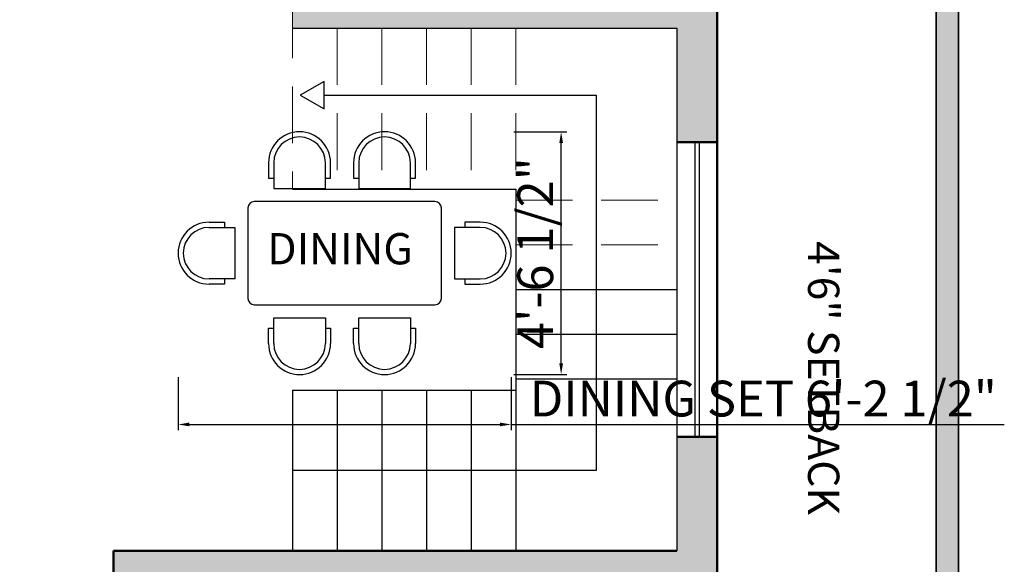
# Model space of a CAD drawing. Units: inches. Extents: x 3008 to 4088, y 1255 to 2137.
# Tile 10 of 30: x 3310 to 3530, y 1665 to 1787. Entities that reach past the tile are written whole.
import ezdxf

# ---------------------------------------------------------------- set-up
doc = ezdxf.new("R2010")
doc.units = ezdxf.units.IN
doc.linetypes.add('DASHED', pattern=[19.05, 12.7, -6.35])
for name, color, linetype, lineweight in [('A-ANNO-DIMS', 2, 'Continuous', 18), ('A-ANNO-TEXT', 7, 'Continuous', 18), ('A-AREA-IDEN', 7, 'Continuous', 18), ('A-FLOR-STRS', 3, 'Continuous', 25), ('A-FLOR-STRS-OVHD', 3, 'DASHED', 18), ('A-FURN', 8, 'Continuous', 18), ('A-GLAZ', 4, 'Continuous', 25), ('A-WALL', 7, 'Continuous', 50), ('A-WALL-PATT', 8, 'Continuous', 13), ('C-PROP', 1, 'Continuous', 35), ('C-PROP-PATT', 9, 'Continuous', 13)]:
    doc.layers.add(name, color=color, linetype=linetype, lineweight=lineweight)
doc.layers.add('NOI THAT', color=42, linetype='Continuous')
doc.styles.get("Standard").update_dxf_attribs({"font": 'arial.ttf'})
doc.dimstyles.new('ISO-25', dxfattribs={"dimtxt": 8, "dimasz": 2.5, "dimexe": 1.25, "dimexo": 0.625, "dimtad": 1, "dimdec": 1, "dimlunit": 3, "dimtxsty": 'Standard', "dimcen": 2.5, "dimadec": 0, "dimazin": 0, "dimtfac": 1, "dimtdec": 1, "dimtmove": 0, "dimatfit": 3, "dimfxl": 1, "dimarcsym": 0})

# ---------------------------------------------------------------- blocks, each defined once
blk = doc.blocks.new('A$C3F0C2877')
at = {"layer": 'NOI THAT'}
for p, q in [((700, 1640), (700, 1520)), ((740, 1640), (740, 1440)), ((1140, 1440), (1140, 1640)), ((1180, 1520), (1180, 1640)), ((1358.3, 1640), (1358.3, 1520)), ((1398.3, 1640), (1398.3, 1440)), ((1798.3, 1440), (1798.3, 1640)), ((1838.3, 1520), (1838.3, 1640)), ((700, 1520), (740, 1520)), ((1140, 1520), (1180, 1520)), ((1358.3, 1520), (1398.3, 1520)), ((1798.3, 1520), (1838.3, 1520)), ((740, 1440), (1140, 1440)), ((1398.3, 1440), (1798.3, 1440)), ((1988.3, 1340), (590, 1340)), ((540, 1290), (540, 590)), ((2038.3, 590), (2038.3, 1290)), ((240, 1180), (360, 1180)), ((360, 1180), (360, 1140)), ((2338.6, 1180), (2218.6, 1180)), ((2218.6, 1180), (2218.6, 1140)), ((240, 1140), (440, 1140)), ((440, 1140), (440, 740)), ((2138.6, 1140), (2138.6, 740)), ((2338.6, 1140), (2138.6, 1140)), ((440, 740), (240, 740)), ((360, 700), (240, 700)), ((360, 740), (360, 700)), ((2138.6, 740), (2338.6, 740)), ((2218.6, 740), (2218.6, 700)), ((2218.6, 700), (2338.6, 700)), ((590, 540), (1988.3, 540)), ((740, 440), (1140, 440)), ((740, 240), (740, 440)), ((1140, 440), (1140, 240)), ((1398.3, 440), (1798.3, 440)), ((1398.3, 240), (1398.3, 440)), ((1798.3, 440), (1798.3, 240)), ((700, 360), (740, 360)), ((700, 240), (700, 360)), ((1140, 360), (1180, 360)), ((1180, 360), (1180, 240)), ((1358.3, 360), (1398.3, 360)), ((1358.3, 240), (1358.3, 360)), ((1798.3, 360), (1838.3, 360)), ((1838.3, 360), (1838.3, 240))]:
    blk.add_line(p, q, dxfattribs=at)
for centre, radius, start, end in [((940, 1640), 240, 0, 180), ((940, 1640), 200, 0, 180), ((1598.3, 1640), 240, 0, 180), ((1598.3, 1640), 200, 0, 180), ((590, 1290), 50, 90, 180), ((1988.3, 1290), 50, 0, 90), ((240, 940), 240, 90, 270), ((2338.6, 940), 240, 270, 90), ((240, 940), 200, 90, 270), ((2338.6, 940), 200, 270, 90), ((590, 590), 50, 180, 270), ((1988.3, 590), 50, 270, 0), ((940, 240), 240, 180, 0), ((940, 240), 200, 180, 0), ((1598.3, 240), 240, 180, 0), ((1598.3, 240), 200, 180, 0)]:
    blk.add_arc(centre, radius, start, end, dxfattribs=at)
blk = doc.blocks.new('*D65')
at = {"layer": 'A-ANNO-DIMS', "color": 0, "lineweight": -2, "transparency": 16777216}
for p, q in [((3345.11, 1706.82), (3345.11, 1695.02)), ((3419.62, 1706.82), (3419.62, 1695.02)), ((3347.61, 1696.27), (3417.12, 1696.27)), ((3419.62, 1696.27), (3529.94, 1696.27))]:
    blk.add_line(p, q, dxfattribs=at)
at = {"layer": 'A-ANNO-DIMS', "color": 0, "transparency": 16777216}
for points in [[(3347.61, 1696.69), (3347.61, 1695.86), (3345.11, 1696.27)], [(3417.12, 1696.69), (3417.12, 1695.86), (3419.62, 1696.27)]]:
    blk.add_solid(points, dxfattribs=at)
at = {"layer": 'Defpoints', "color": 0, "transparency": 16777216}
for p in [(3345.11, 1707.45), (3419.62, 1707.45), (3419.62, 1696.27)]:
    blk.add_point(p, dxfattribs=at)
at = {"layer": 'A-ANNO-DIMS', "color": 0, "transparency": 16777216, "insert": (3476.03, 1701.03), "char_height": 8, "attachment_point": 5}
blk.add_mtext('DINING SET 6\'-2 1/2"', dxfattribs=at)
blk = doc.blocks.new('*D66')
at = {"layer": 'A-ANNO-DIMS', "color": 0, "lineweight": -2, "transparency": 16777216}
for p, q in [((3420.25, 1761.77), (3432.05, 1761.77)), ((3430.8, 1709.95), (3430.8, 1759.27)), ((3420.25, 1707.45), (3432.05, 1707.45))]:
    blk.add_line(p, q, dxfattribs=at)
at = {"layer": 'A-ANNO-DIMS', "color": 0, "transparency": 16777216}
for points in [[(3430.38, 1759.27), (3431.21, 1759.27), (3430.8, 1761.77)], [(3430.38, 1709.95), (3431.21, 1709.95), (3430.8, 1707.45)]]:
    blk.add_solid(points, dxfattribs=at)
at = {"layer": 'Defpoints', "color": 0, "transparency": 16777216}
for p in [(3419.62, 1761.77), (3430.8, 1761.77), (3419.62, 1707.45)]:
    blk.add_point(p, dxfattribs=at)
at = {"layer": 'A-ANNO-DIMS', "color": 0, "transparency": 16777216, "insert": (3426.04, 1734.61), "char_height": 8, "attachment_point": 5, "rotation": 90}
blk.add_mtext('4\'-6 1/2"', dxfattribs=at)

msp = doc.modelspace()

# ---------------------------------------------------------------- hatches: boundary and pattern name
at = {"layer": 'A-WALL-PATT'}
h = msp.add_hatch(color=256, dxfattribs=at)
h.dxf.hatch_style = 1
h.paths.add_polyline_path([(3102.67, 1625.97), (3093.67, 1625.97), (3093.67, 1540.97), (3102.67, 1540.97)])
h.paths.add_polyline_path([(3102.67, 1784.97), (3252.67, 1784.97), (3252.67, 1790.97), (3102.67, 1790.97), (3102.67, 1892.97), (3093.67, 1892.97), (3093.67, 1667.97), (3102.67, 1667.97)])
h.paths.add_polyline_path([(3192.67, 1943.97), (3093.67, 1943.97), (3093.67, 1934.97), (3102.67, 1934.97), (3192.67, 1934.97)])
h.paths.add_polyline_path([(3264.67, 1943.97), (3234.67, 1943.97), (3234.67, 1934.97), (3246.67, 1934.97), (3246.67, 1868.97), (3252.67, 1868.97), (3252.67, 1934.97), (3264.67, 1934.97)])
h.paths.add_polyline_path([(3330.67, 1943.97), (3288.67, 1943.97), (3288.67, 1934.97), (3300.67, 1934.97), (3300.67, 1838.97), (3246.67, 1838.97), (3246.67, 1826.97), (3252.67, 1826.97), (3252.67, 1832.97), (3306.67, 1832.97), (3306.67, 1934.97), (3330.67, 1934.97)])
h.paths.add_polyline_path([(3390.67, 1943.97), (3360.67, 1943.97), (3360.67, 1934.97), (3390.67, 1934.97)])
h.paths.add_polyline_path([(3465.67, 1943.97), (3432.67, 1943.97), (3432.67, 1934.97), (3456.67, 1934.97), (3456.67, 1883.97), (3465.67, 1883.97)])
h.paths.add_polyline_path([(3465.67, 1841.97), (3456.67, 1841.97), (3456.67, 1790.97), (3370.67, 1790.97), (3370.67, 1784.97), (3456.67, 1784.97), (3456.67, 1759.47), (3465.67, 1759.47)])
h.paths.add_polyline_path([(3465.67, 1693.47), (3456.67, 1693.47), (3456.67, 1667.97), (3330.67, 1667.97), (3330.67, 1643.97), (3336.67, 1643.97), (3336.67, 1661.97), (3456.67, 1661.97), (3456.67, 1649.97), (3465.67, 1649.97)])
h.paths.add_polyline_path([(3465.67, 1625.97), (3456.67, 1625.97), (3456.67, 1613.97), (3324.67, 1613.97), (3324.67, 1604.97), (3456.67, 1604.97), (3456.67, 1571.97), (3465.67, 1571.97)])
h.paths.add_polyline_path([(3465.67, 1505.97), (3456.67, 1505.97), (3456.67, 1472.97), (3438.67, 1472.97), (3438.67, 1463.97), (3465.67, 1463.97)])
h.paths.add_polyline_path([(3396.67, 1472.97), (3354.67, 1472.97), (3354.67, 1463.97), (3396.67, 1463.97)])
h.paths.add_polyline_path([(3312.67, 1472.97), (3288.67, 1472.97), (3288.67, 1550.97), (3282.67, 1550.97), (3282.67, 1472.97), (3270.67, 1472.97), (3270.67, 1463.97), (3312.67, 1463.97)])
h.paths.add_polyline_path([(3246.67, 1472.97), (3234.67, 1472.97), (3234.67, 1544.97), (3252.67, 1544.97), (3252.67, 1550.97), (3234.67, 1550.97), (3234.67, 1604.97), (3282.67, 1604.97), (3282.67, 1580.97), (3288.67, 1580.97), (3288.67, 1613.97), (3150.67, 1613.97), (3150.67, 1604.97), (3225.67, 1604.97), (3225.67, 1463.97), (3246.67, 1463.97)])
at = {"layer": 'C-PROP-PATT'}
h = msp.add_hatch(color=256, dxfattribs=at)
h.dxf.hatch_style = 1
h.paths.add_polyline_path([(3519.67, 2003.97), (3039.67, 2003.97), (3039.67, 1343.97), (3051.67, 1343.97), (3051.67, 1348.97), (3044.67, 1348.97), (3044.67, 1998.97), (3514.67, 1998.97), (3514.67, 1348.97), (3219.67, 1348.97), (3219.67, 1343.97), (3519.67, 1343.97)])

# ---------------------------------------------------------------- linework, layer by layer
at = {"layer": 'A-FLOR-STRS'}
for p, q in [((3370.67, 1784.97), (3456.67, 1784.97)), ((3456.67, 1784.97), (3456.67, 1667.97)), ((3370.67, 1748.97), (3420.67, 1748.97)), ((3420.67, 1748.97), (3420.67, 1667.97)), ((3420.67, 1726.47), (3456.67, 1726.47)), ((3420.67, 1716.47), (3456.67, 1716.47)), ((3420.67, 1706.47), (3456.67, 1706.47)), ((3370.67, 1703.97), (3420.67, 1703.97)), ((3370.67, 1703.97), (3370.67, 1667.97)), ((3380.67, 1703.97), (3380.67, 1667.97)), ((3390.67, 1703.97), (3390.67, 1667.97)), ((3400.67, 1703.97), (3400.67, 1667.97)), ((3410.67, 1703.97), (3410.67, 1667.97))]:
    msp.add_line(p, q, dxfattribs=at)
msp.add_lwpolyline([(3372.45, 1769.97), (3377.8, 1766.88), (3377.8, 1773.06)], close=True, dxfattribs=at)
msp.add_lwpolyline([(3377.8, 1769.97), (3438.67, 1769.97), (3438.67, 1685.97), (3370.67, 1685.97)], dxfattribs=at)
at = {"layer": 'A-FLOR-STRS-OVHD'}
for p, q in [((3370.67, 1790.97), (3370.67, 1748.97)), ((3380.67, 1784.97), (3380.67, 1748.97)), ((3390.67, 1784.97), (3390.67, 1748.97)), ((3400.67, 1784.97), (3400.67, 1748.97)), ((3410.67, 1784.97), (3410.67, 1748.97)), ((3420.67, 1784.97), (3420.67, 1748.97)), ((3420.67, 1746.47), (3456.67, 1746.47)), ((3420.67, 1736.47), (3456.67, 1736.47))]:
    msp.add_line(p, q, dxfattribs=at)
at = {"layer": 'A-GLAZ'}
for p, q in [((3460.67, 1759.47), (3460.67, 1693.47)), ((3460.67, 1759.47), (3460.67, 1693.47)), ((3461.67, 1759.47), (3461.67, 1693.47))]:
    msp.add_line(p, q, dxfattribs=at)
at = {"layer": 'A-WALL'}
for p, q in [((3465.67, 1998.97), (3465.67, 1463.97)), ((3456.67, 1759.47), (3465.67, 1759.47)), ((3456.67, 1693.47), (3465.67, 1693.47)), ((3330.67, 1667.97), (3456.67, 1667.97)), ((3330.67, 1667.97), (3330.67, 1643.97))]:
    msp.add_line(p, q, dxfattribs=at)
at = {"layer": 'C-PROP'}
for p, q in [((3519.67, 2003.97), (3519.67, 1343.97)), ((3514.67, 1998.97), (3514.67, 1348.97))]:
    msp.add_line(p, q, dxfattribs=at)

# ---------------------------------------------------------------- block references
at = {"layer": 'A-FURN', "xscale": 0.0288952394299788, "yscale": 0.0288952394299788, "zscale": 0.0288952394299788}
msp.add_blockref('A$C3F0C2877', (3345.11, 1707.45), dxfattribs=at)

# ---------------------------------------------------------------- texts
at = {"layer": 'A-ANNO-TEXT', "insert": (3493.03, 1737.31), "char_height": 7, "attachment_point": 1, "rotation": 270}
msp.add_mtext_dynamic_manual_height_columns('{\\fTimes New Roman|b0|i0|c0|p18;4\'6" SETBACK}', width=105.6127, gutter_width=12.5, heights=[0], dxfattribs=at)
at = {"layer": 'A-AREA-IDEN', "insert": (3365.05, 1739.11), "char_height": 7, "attachment_point": 1}
msp.add_mtext_dynamic_manual_height_columns('{\\fTimes New Roman|b0|i0|c0|p18;DINING}', width=105.6127, gutter_width=12.5, heights=[0], dxfattribs=at)

# ---------------------------------------------------------------- dimensions: what is measured, and where the dimension line sits
at = {"layer": 'A-ANNO-DIMS'}
dim = msp.add_linear_dim(base=(3430.8, 1761.77), p1=(3419.62, 1707.45), p2=(3419.62, 1761.77), angle=90, dimstyle='ISO-25', override={"dimdec": 1, "dimrnd": 0, "dimzin": 1, "dimlunit": 4, "dimfrac": 2}, dxfattribs=at)
dim.commit()
dim.dimension.update_dxf_attribs({"geometry": '*D66', "text_midpoint": (3426.04, 1734.61)})
dim = msp.add_linear_dim(base=(3419.62, 1696.27), p1=(3345.11, 1707.45), p2=(3419.62, 1707.45), text='DINING SET <>', dimstyle='ISO-25', override={"dimdec": 1, "dimrnd": 0, "dimzin": 1, "dimlunit": 4, "dimfrac": 2}, dxfattribs=at)
dim.commit()
dim.dimension.update_dxf_attribs({"geometry": '*D65', "text_midpoint": (3476.03, 1701.03)})

doc.saveas('drawing.dxf')
